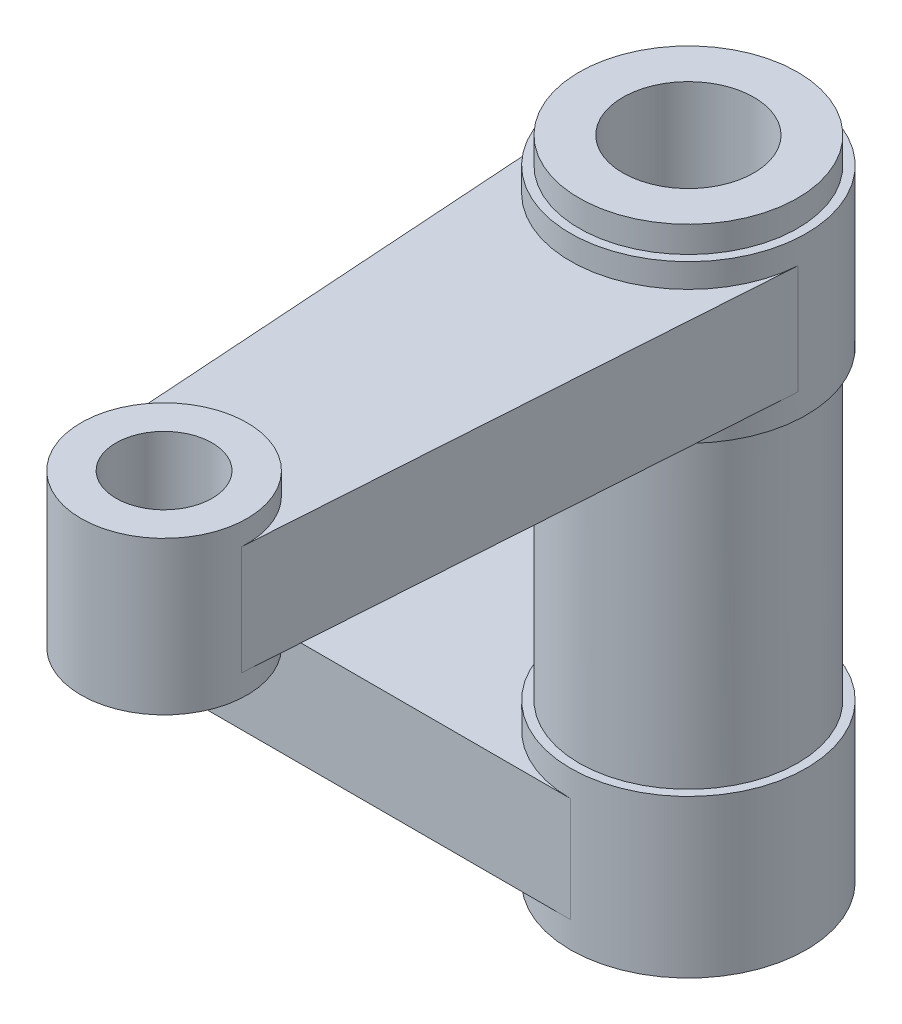
ISO-10303-21;
HEADER;
FILE_DESCRIPTION(('STEP AP214'),'2;1');
FILE_NAME('part.step','',(''),(''),'','','');
FILE_SCHEMA(('AUTOMOTIVE_DESIGN { 1 0 10303 214 1 1 1 1 }'));
ENDSEC;
DATA;
#1=APPLICATION_CONTEXT('core data for automotive mechanical design processes');
#2=APPLICATION_PROTOCOL_DEFINITION('international standard','automotive_design',2000,#1);
#3=PRODUCT_CONTEXT('',#1,'mechanical');
#4=PRODUCT('Part','Part','',(#3));
#5=PRODUCT_RELATED_PRODUCT_CATEGORY('part','',(#4));
#6=PRODUCT_DEFINITION_FORMATION('','',#4);
#7=PRODUCT_DEFINITION_CONTEXT('part definition',#1,'design');
#8=PRODUCT_DEFINITION('design','',#6,#7);
#9=PRODUCT_DEFINITION_SHAPE('','',#8);
#10=(LENGTH_UNIT() NAMED_UNIT(*) SI_UNIT(.MILLI.,.METRE.));
#11=(NAMED_UNIT(*) PLANE_ANGLE_UNIT() SI_UNIT($,.RADIAN.));
#12=(NAMED_UNIT(*) SI_UNIT($,.STERADIAN.) SOLID_ANGLE_UNIT());
#13=UNCERTAINTY_MEASURE_WITH_UNIT(LENGTH_MEASURE(1.E-05),#10,'distance_accuracy_value','');
#14=(GEOMETRIC_REPRESENTATION_CONTEXT(3) GLOBAL_UNCERTAINTY_ASSIGNED_CONTEXT((#13)) GLOBAL_UNIT_ASSIGNED_CONTEXT((#10,
#11,#12)) REPRESENTATION_CONTEXT('',''));
#15=CARTESIAN_POINT('',(0.,0.,0.));
#16=DIRECTION('',(0.,0.,1.));
#17=DIRECTION('',(1.,0.,0.));
#18=AXIS2_PLACEMENT_3D('',#15,#16,#17);
#19=CARTESIAN_POINT('',(-45.,6.,0.));
#20=DIRECTION('',(0.,1.,0.));
#21=DIRECTION('',(0.,0.,1.));
#22=AXIS2_PLACEMENT_3D('',#19,#20,#21);
#23=PLANE('',#22);
#24=CARTESIAN_POINT('',(-45.,6.,0.));
#25=DIRECTION('',(0.,1.,0.));
#26=DIRECTION('',(0.,0.,1.));
#27=AXIS2_PLACEMENT_3D('',#24,#25,#26);
#28=CIRCLE('',#27,7.5);
#29=CARTESIAN_POINT('',(-45.,6.,7.50000000000001));
#30=VERTEX_POINT('',#29);
#31=EDGE_CURVE('E177',#30,#30,#28,.T.);
#32=ORIENTED_EDGE('',*,*,#31,.F.);
#33=EDGE_LOOP('',(#32));
#34=FACE_BOUND('',#33,.T.);
#35=DIRECTION('',(1.,0.,0.));
#36=VECTOR('',#35,1.);
#37=CARTESIAN_POINT('',(-45.,6.,13.5));
#38=LINE('',#37,#36);
#39=CARTESIAN_POINT('',(-45.,6.,13.5));
#40=VERTEX_POINT('',#39);
#41=CARTESIAN_POINT('',(0.,6.,13.5));
#42=VERTEX_POINT('',#41);
#43=EDGE_CURVE('E87',#40,#42,#38,.T.);
#44=ORIENTED_EDGE('',*,*,#43,.T.);
#45=CARTESIAN_POINT('',(0.,6.,0.));
#46=DIRECTION('',(0.,1.,0.));
#47=DIRECTION('',(0.,0.,1.));
#48=AXIS2_PLACEMENT_3D('',#45,#46,#47);
#49=CIRCLE('',#48,13.5);
#50=CARTESIAN_POINT('',(0.,6.,-13.5));
#51=VERTEX_POINT('',#50);
#52=EDGE_CURVE('E180',#42,#51,#49,.F.);
#53=ORIENTED_EDGE('',*,*,#52,.T.);
#54=DIRECTION('',(-1.,0.,0.));
#55=VECTOR('',#54,1.);
#56=CARTESIAN_POINT('',(-45.,6.,-13.5));
#57=LINE('',#56,#55);
#58=CARTESIAN_POINT('',(-45.,6.,-13.5));
#59=VERTEX_POINT('',#58);
#60=EDGE_CURVE('E64',#51,#59,#57,.T.);
#61=ORIENTED_EDGE('',*,*,#60,.T.);
#62=CARTESIAN_POINT('',(-45.,6.,0.));
#63=DIRECTION('',(0.,1.,0.));
#64=DIRECTION('',(0.,0.,1.));
#65=AXIS2_PLACEMENT_3D('',#62,#63,#64);
#66=CIRCLE('',#65,13.5);
#67=EDGE_CURVE('E186',#59,#40,#66,.T.);
#68=ORIENTED_EDGE('',*,*,#67,.T.);
#69=EDGE_LOOP('',(#44,#53,#61,#68));
#70=FACE_BOUND('',#69,.T.);
#71=ADVANCED_FACE('F39',(#34,#70),#23,.T.);
#72=CARTESIAN_POINT('',(-45.,-6.,0.));
#73=DIRECTION('',(0.,1.,0.));
#74=DIRECTION('',(0.,0.,1.));
#75=AXIS2_PLACEMENT_3D('',#72,#73,#74);
#76=PLANE('',#75);
#77=CARTESIAN_POINT('',(-45.,-6.,0.));
#78=DIRECTION('',(0.,1.,0.));
#79=DIRECTION('',(0.,0.,1.));
#80=AXIS2_PLACEMENT_3D('',#77,#78,#79);
#81=CIRCLE('',#80,7.5);
#82=CARTESIAN_POINT('',(-45.,-6.,7.50000000000001));
#83=VERTEX_POINT('',#82);
#84=EDGE_CURVE('E179',#83,#83,#81,.T.);
#85=ORIENTED_EDGE('',*,*,#84,.T.);
#86=EDGE_LOOP('',(#85));
#87=FACE_BOUND('',#86,.T.);
#88=CARTESIAN_POINT('',(0.,-6.,0.));
#89=DIRECTION('',(0.,1.,0.));
#90=DIRECTION('',(0.,0.,1.));
#91=AXIS2_PLACEMENT_3D('',#88,#89,#90);
#92=CIRCLE('',#91,13.5);
#93=CARTESIAN_POINT('',(0.,-6.,13.5));
#94=VERTEX_POINT('',#93);
#95=CARTESIAN_POINT('',(0.,-6.,-13.5));
#96=VERTEX_POINT('',#95);
#97=EDGE_CURVE('E174',#94,#96,#92,.F.);
#98=ORIENTED_EDGE('',*,*,#97,.F.);
#99=DIRECTION('',(1.,0.,0.));
#100=VECTOR('',#99,1.);
#101=CARTESIAN_POINT('',(-45.,-6.,13.5));
#102=LINE('',#101,#100);
#103=CARTESIAN_POINT('',(-45.,-6.,13.5));
#104=VERTEX_POINT('',#103);
#105=EDGE_CURVE('E191',#104,#94,#102,.T.);
#106=ORIENTED_EDGE('',*,*,#105,.F.);
#107=CARTESIAN_POINT('',(-45.,-6.,0.));
#108=DIRECTION('',(0.,1.,0.));
#109=DIRECTION('',(0.,0.,1.));
#110=AXIS2_PLACEMENT_3D('',#107,#108,#109);
#111=CIRCLE('',#110,13.5);
#112=CARTESIAN_POINT('',(-45.,-6.,-13.5));
#113=VERTEX_POINT('',#112);
#114=EDGE_CURVE('E181',#113,#104,#111,.T.);
#115=ORIENTED_EDGE('',*,*,#114,.F.);
#116=DIRECTION('',(-1.,0.,0.));
#117=VECTOR('',#116,1.);
#118=CARTESIAN_POINT('',(-45.,-6.,-13.5));
#119=LINE('',#118,#117);
#120=EDGE_CURVE('E83',#96,#113,#119,.T.);
#121=ORIENTED_EDGE('',*,*,#120,.F.);
#122=EDGE_LOOP('',(#98,#106,#115,#121));
#123=FACE_BOUND('',#122,.T.);
#124=ADVANCED_FACE('F208',(#87,#123),#76,.F.);
#125=CARTESIAN_POINT('',(-45.,6.,0.));
#126=DIRECTION('',(0.,-1.,0.));
#127=DIRECTION('',(0.,0.,-1.));
#128=AXIS2_PLACEMENT_3D('',#125,#126,#127);
#129=CYLINDRICAL_SURFACE('',#128,13.5);
#130=ORIENTED_EDGE('',*,*,#114,.T.);
#131=DIRECTION('',(0.,-1.,0.));
#132=VECTOR('',#131,1.);
#133=CARTESIAN_POINT('',(-45.,6.,13.5));
#134=LINE('',#133,#132);
#135=EDGE_CURVE('E50',#40,#104,#134,.T.);
#136=ORIENTED_EDGE('',*,*,#135,.F.);
#137=ORIENTED_EDGE('',*,*,#67,.F.);
#138=DIRECTION('',(0.,-1.,0.));
#139=VECTOR('',#138,1.);
#140=CARTESIAN_POINT('',(-45.,6.,-13.5));
#141=LINE('',#140,#139);
#142=EDGE_CURVE('E190',#59,#113,#141,.T.);
#143=ORIENTED_EDGE('',*,*,#142,.T.);
#144=EDGE_LOOP('',(#130,#136,#137,#143));
#145=FACE_BOUND('',#144,.T.);
#146=ADVANCED_FACE('F41',(#145),#129,.T.);
#147=CARTESIAN_POINT('',(-45.,6.,13.5));
#148=DIRECTION('',(0.,0.,-1.));
#149=DIRECTION('',(-1.,0.,0.));
#150=AXIS2_PLACEMENT_3D('',#147,#148,#149);
#151=PLANE('',#150);
#152=ORIENTED_EDGE('',*,*,#105,.T.);
#153=DIRECTION('',(0.,-1.,0.));
#154=VECTOR('',#153,1.);
#155=CARTESIAN_POINT('',(0.,6.,13.5));
#156=LINE('',#155,#154);
#157=EDGE_CURVE('E199',#42,#94,#156,.T.);
#158=ORIENTED_EDGE('',*,*,#157,.F.);
#159=ORIENTED_EDGE('',*,*,#43,.F.);
#160=ORIENTED_EDGE('',*,*,#135,.T.);
#161=EDGE_LOOP('',(#152,#158,#159,#160));
#162=FACE_BOUND('',#161,.T.);
#163=ADVANCED_FACE('F201',(#162),#151,.F.);
#164=CARTESIAN_POINT('',(0.,6.,0.));
#165=DIRECTION('',(0.,-1.,0.));
#166=DIRECTION('',(0.,0.,-1.));
#167=AXIS2_PLACEMENT_3D('',#164,#165,#166);
#168=CYLINDRICAL_SURFACE('',#167,13.5);
#169=ORIENTED_EDGE('',*,*,#157,.T.);
#170=ORIENTED_EDGE('',*,*,#97,.T.);
#171=DIRECTION('',(0.,-1.,0.));
#172=VECTOR('',#171,1.);
#173=CARTESIAN_POINT('',(0.,6.,-13.5));
#174=LINE('',#173,#172);
#175=EDGE_CURVE('E196',#51,#96,#174,.T.);
#176=ORIENTED_EDGE('',*,*,#175,.F.);
#177=ORIENTED_EDGE('',*,*,#52,.F.);
#178=EDGE_LOOP('',(#169,#170,#176,#177));
#179=FACE_BOUND('',#178,.T.);
#180=CARTESIAN_POINT('',(0.,-9.,0.));
#181=DIRECTION('',(0.,1.,0.));
#182=DIRECTION('',(0.,0.,1.));
#183=AXIS2_PLACEMENT_3D('',#180,#181,#182);
#184=CIRCLE('',#183,13.5);
#185=CARTESIAN_POINT('',(0.,-9.,13.5));
#186=VERTEX_POINT('',#185);
#187=EDGE_CURVE('E166',#186,#186,#184,.T.);
#188=ORIENTED_EDGE('',*,*,#187,.T.);
#189=EDGE_LOOP('',(#188));
#190=FACE_BOUND('',#189,.T.);
#191=CARTESIAN_POINT('',(0.,9.,0.));
#192=DIRECTION('',(0.,1.,0.));
#193=DIRECTION('',(0.,0.,1.));
#194=AXIS2_PLACEMENT_3D('',#191,#192,#193);
#195=CIRCLE('',#194,13.5);
#196=CARTESIAN_POINT('',(0.,9.,13.5));
#197=VERTEX_POINT('',#196);
#198=EDGE_CURVE('E168',#197,#197,#195,.T.);
#199=ORIENTED_EDGE('',*,*,#198,.F.);
#200=EDGE_LOOP('',(#199));
#201=FACE_BOUND('',#200,.T.);
#202=ADVANCED_FACE('F211',(#179,#190,#201),#168,.T.);
#203=CARTESIAN_POINT('',(-45.,6.,-13.5));
#204=DIRECTION('',(0.,0.,1.));
#205=DIRECTION('',(1.,0.,0.));
#206=AXIS2_PLACEMENT_3D('',#203,#204,#205);
#207=PLANE('',#206);
#208=ORIENTED_EDGE('',*,*,#120,.T.);
#209=ORIENTED_EDGE('',*,*,#142,.F.);
#210=ORIENTED_EDGE('',*,*,#60,.F.);
#211=ORIENTED_EDGE('',*,*,#175,.T.);
#212=EDGE_LOOP('',(#208,#209,#210,#211));
#213=FACE_BOUND('',#212,.T.);
#214=ADVANCED_FACE('F212',(#213),#207,.F.);
#215=CARTESIAN_POINT('',(-45.,6.,0.));
#216=DIRECTION('',(0.,-1.,0.));
#217=DIRECTION('',(0.,0.,-1.));
#218=AXIS2_PLACEMENT_3D('',#215,#216,#217);
#219=CYLINDRICAL_SURFACE('',#218,7.5);
#220=ORIENTED_EDGE('',*,*,#31,.T.);
#221=EDGE_LOOP('',(#220));
#222=FACE_BOUND('',#221,.T.);
#223=ORIENTED_EDGE('',*,*,#84,.F.);
#224=EDGE_LOOP('',(#223));
#225=FACE_BOUND('',#224,.T.);
#226=ADVANCED_FACE('F226',(#222,#225),#219,.F.);
#227=CARTESIAN_POINT('',(0.,-9.,0.));
#228=DIRECTION('',(0.,1.,0.));
#229=DIRECTION('',(0.,0.,1.));
#230=AXIS2_PLACEMENT_3D('',#227,#228,#229);
#231=PLANE('',#230);
#232=CARTESIAN_POINT('',(0.,-8.99999999999999,0.));
#233=DIRECTION('',(0.,1.,0.));
#234=DIRECTION('',(0.,0.,1.));
#235=AXIS2_PLACEMENT_3D('',#232,#233,#234);
#236=CIRCLE('',#235,7.5);
#237=CARTESIAN_POINT('',(0.,-8.99999999999999,7.5));
#238=VERTEX_POINT('',#237);
#239=EDGE_CURVE('E149',#238,#238,#236,.T.);
#240=ORIENTED_EDGE('',*,*,#239,.T.);
#241=EDGE_LOOP('',(#240));
#242=FACE_BOUND('',#241,.T.);
#243=ORIENTED_EDGE('',*,*,#187,.F.);
#244=EDGE_LOOP('',(#243));
#245=FACE_BOUND('',#244,.T.);
#246=ADVANCED_FACE('F244',(#242,#245),#231,.F.);
#247=CARTESIAN_POINT('',(0.,9.,0.));
#248=DIRECTION('',(0.,1.,0.));
#249=DIRECTION('',(0.,0.,1.));
#250=AXIS2_PLACEMENT_3D('',#247,#248,#249);
#251=PLANE('',#250);
#252=CARTESIAN_POINT('',(0.,9.,0.));
#253=DIRECTION('',(0.,1.,0.));
#254=DIRECTION('',(0.,0.,1.));
#255=AXIS2_PLACEMENT_3D('',#252,#253,#254);
#256=CIRCLE('',#255,12.5);
#257=CARTESIAN_POINT('',(0.,9.,12.5));
#258=VERTEX_POINT('',#257);
#259=EDGE_CURVE('E11',#258,#258,#256,.T.);
#260=ORIENTED_EDGE('',*,*,#259,.F.);
#261=EDGE_LOOP('',(#260));
#262=FACE_BOUND('',#261,.T.);
#263=ORIENTED_EDGE('',*,*,#198,.T.);
#264=EDGE_LOOP('',(#263));
#265=FACE_BOUND('',#264,.T.);
#266=ADVANCED_FACE('F277',(#262,#265),#251,.T.);
#267=CARTESIAN_POINT('',(0.,65.,0.));
#268=DIRECTION('',(0.,1.,0.));
#269=DIRECTION('',(0.,0.,1.));
#270=AXIS2_PLACEMENT_3D('',#267,#268,#269);
#271=PLANE('',#270);
#272=CARTESIAN_POINT('',(0.,65.,0.));
#273=DIRECTION('',(0.,1.,0.));
#274=DIRECTION('',(0.,0.,1.));
#275=AXIS2_PLACEMENT_3D('',#272,#273,#274);
#276=CIRCLE('',#275,7.5);
#277=CARTESIAN_POINT('',(0.,65.,7.5));
#278=VERTEX_POINT('',#277);
#279=EDGE_CURVE('E146',#278,#278,#276,.T.);
#280=ORIENTED_EDGE('',*,*,#279,.F.);
#281=EDGE_LOOP('',(#280));
#282=FACE_BOUND('',#281,.T.);
#283=CARTESIAN_POINT('',(0.,65.,0.));
#284=DIRECTION('',(0.,-1.,0.));
#285=DIRECTION('',(0.,0.,-1.));
#286=AXIS2_PLACEMENT_3D('',#283,#284,#285);
#287=CIRCLE('',#286,12.5);
#288=CARTESIAN_POINT('',(0.,65.,-12.5));
#289=VERTEX_POINT('',#288);
#290=EDGE_CURVE('E167',#289,#289,#287,.T.);
#291=ORIENTED_EDGE('',*,*,#290,.F.);
#292=EDGE_LOOP('',(#291));
#293=FACE_BOUND('',#292,.T.);
#294=ADVANCED_FACE('F290',(#282,#293),#271,.T.);
#295=CARTESIAN_POINT('',(0.,0.,0.));
#296=DIRECTION('',(0.,-1.,0.));
#297=DIRECTION('',(0.,0.,-1.));
#298=AXIS2_PLACEMENT_3D('',#295,#296,#297);
#299=CYLINDRICAL_SURFACE('',#298,12.5);
#300=ORIENTED_EDGE('',*,*,#290,.T.);
#301=EDGE_LOOP('',(#300));
#302=FACE_BOUND('',#301,.T.);
#303=CARTESIAN_POINT('',(0.,62.,0.));
#304=DIRECTION('',(0.,-1.,0.));
#305=DIRECTION('',(0.,0.,-1.));
#306=AXIS2_PLACEMENT_3D('',#303,#304,#305);
#307=CIRCLE('',#306,12.5);
#308=CARTESIAN_POINT('',(0.,62.,-12.5));
#309=VERTEX_POINT('',#308);
#310=EDGE_CURVE('E162',#309,#309,#307,.T.);
#311=ORIENTED_EDGE('',*,*,#310,.F.);
#312=EDGE_LOOP('',(#311));
#313=FACE_BOUND('',#312,.T.);
#314=ADVANCED_FACE('F297',(#302,#313),#299,.T.);
#315=CARTESIAN_POINT('',(12.5,62.,0.));
#316=DIRECTION('',(0.,1.,0.));
#317=DIRECTION('',(0.,0.,1.));
#318=AXIS2_PLACEMENT_3D('',#315,#316,#317);
#319=PLANE('',#318);
#320=ORIENTED_EDGE('',*,*,#310,.T.);
#321=EDGE_LOOP('',(#320));
#322=FACE_BOUND('',#321,.T.);
#323=CARTESIAN_POINT('',(0.,62.,0.));
#324=DIRECTION('',(0.,-1.,0.));
#325=DIRECTION('',(0.,0.,-1.));
#326=AXIS2_PLACEMENT_3D('',#323,#324,#325);
#327=CIRCLE('',#326,13.5);
#328=CARTESIAN_POINT('',(0.,62.,-13.5));
#329=VERTEX_POINT('',#328);
#330=EDGE_CURVE('E159',#329,#329,#327,.T.);
#331=ORIENTED_EDGE('',*,*,#330,.F.);
#332=EDGE_LOOP('',(#331));
#333=FACE_BOUND('',#332,.T.);
#334=ADVANCED_FACE('F307',(#322,#333),#319,.T.);
#335=CARTESIAN_POINT('',(0.,0.,0.));
#336=DIRECTION('',(0.,-1.,0.));
#337=DIRECTION('',(0.,0.,-1.));
#338=AXIS2_PLACEMENT_3D('',#335,#336,#337);
#339=CYLINDRICAL_SURFACE('',#338,13.5);
#340=CARTESIAN_POINT('',(0.,59.25,0.));
#341=DIRECTION('',(0.,-1.,0.));
#342=DIRECTION('',(0.,0.,1.));
#343=AXIS2_PLACEMENT_3D('',#340,#341,#342);
#344=CIRCLE('',#343,13.5);
#345=CARTESIAN_POINT('',(13.4699665923862,59.25,0.899999999999999));
#346=VERTEX_POINT('',#345);
#347=CARTESIAN_POINT('',(-13.4699665923862,59.25,0.900000000000002));
#348=VERTEX_POINT('',#347);
#349=EDGE_CURVE('E122',#346,#348,#344,.T.);
#350=ORIENTED_EDGE('',*,*,#349,.F.);
#351=DIRECTION('',(0.,-1.,0.));
#352=VECTOR('',#351,1.);
#353=CARTESIAN_POINT('',(13.4699665923862,59.25,0.899999999999999));
#354=LINE('',#353,#352);
#355=CARTESIAN_POINT('',(13.4699665923862,46.75,0.899999999999999));
#356=VERTEX_POINT('',#355);
#357=EDGE_CURVE('E135',#346,#356,#354,.T.);
#358=ORIENTED_EDGE('',*,*,#357,.T.);
#359=CARTESIAN_POINT('',(0.,46.75,0.));
#360=DIRECTION('',(0.,-1.,0.));
#361=DIRECTION('',(0.,0.,1.));
#362=AXIS2_PLACEMENT_3D('',#359,#360,#361);
#363=CIRCLE('',#362,13.5);
#364=CARTESIAN_POINT('',(-13.4699665923862,46.75,0.900000000000002));
#365=VERTEX_POINT('',#364);
#366=EDGE_CURVE('E123',#356,#365,#363,.T.);
#367=ORIENTED_EDGE('',*,*,#366,.T.);
#368=DIRECTION('',(0.,-1.,0.));
#369=VECTOR('',#368,1.);
#370=CARTESIAN_POINT('',(-13.4699665923862,59.25,0.900000000000002));
#371=LINE('',#370,#369);
#372=EDGE_CURVE('E53',#348,#365,#371,.T.);
#373=ORIENTED_EDGE('',*,*,#372,.F.);
#374=EDGE_LOOP('',(#350,#358,#367,#373));
#375=FACE_BOUND('',#374,.T.);
#376=ORIENTED_EDGE('',*,*,#330,.T.);
#377=EDGE_LOOP('',(#376));
#378=FACE_BOUND('',#377,.T.);
#379=CARTESIAN_POINT('',(0.,44.,0.));
#380=DIRECTION('',(0.,-1.,0.));
#381=DIRECTION('',(0.,0.,-1.));
#382=AXIS2_PLACEMENT_3D('',#379,#380,#381);
#383=CIRCLE('',#382,13.5);
#384=CARTESIAN_POINT('',(0.,44.,-13.5));
#385=VERTEX_POINT('',#384);
#386=EDGE_CURVE('E160',#385,#385,#383,.T.);
#387=ORIENTED_EDGE('',*,*,#386,.F.);
#388=EDGE_LOOP('',(#387));
#389=FACE_BOUND('',#388,.T.);
#390=ADVANCED_FACE('F320',(#375,#378,#389),#339,.T.);
#391=CARTESIAN_POINT('',(13.5,44.,0.));
#392=DIRECTION('',(0.,-1.,0.));
#393=DIRECTION('',(0.,0.,-1.));
#394=AXIS2_PLACEMENT_3D('',#391,#392,#393);
#395=PLANE('',#394);
#396=ORIENTED_EDGE('',*,*,#386,.T.);
#397=EDGE_LOOP('',(#396));
#398=FACE_BOUND('',#397,.T.);
#399=CARTESIAN_POINT('',(0.,44.,0.));
#400=DIRECTION('',(0.,-1.,0.));
#401=DIRECTION('',(0.,0.,-1.));
#402=AXIS2_PLACEMENT_3D('',#399,#400,#401);
#403=CIRCLE('',#402,12.5);
#404=CARTESIAN_POINT('',(0.,44.,-12.5));
#405=VERTEX_POINT('',#404);
#406=EDGE_CURVE('E155',#405,#405,#403,.T.);
#407=ORIENTED_EDGE('',*,*,#406,.F.);
#408=EDGE_LOOP('',(#407));
#409=FACE_BOUND('',#408,.T.);
#410=ADVANCED_FACE('F327',(#398,#409),#395,.T.);
#411=CARTESIAN_POINT('',(0.,0.,0.));
#412=DIRECTION('',(0.,-1.,0.));
#413=DIRECTION('',(0.,0.,-1.));
#414=AXIS2_PLACEMENT_3D('',#411,#412,#413);
#415=CYLINDRICAL_SURFACE('',#414,12.5);
#416=ORIENTED_EDGE('',*,*,#259,.T.);
#417=EDGE_LOOP('',(#416));
#418=FACE_BOUND('',#417,.T.);
#419=ORIENTED_EDGE('',*,*,#406,.T.);
#420=EDGE_LOOP('',(#419));
#421=FACE_BOUND('',#420,.T.);
#422=ADVANCED_FACE('F339',(#418,#421),#415,.T.);
#423=CARTESIAN_POINT('',(0.,-8.99999999999999,0.));
#424=DIRECTION('',(0.,1.,0.));
#425=DIRECTION('',(0.,0.,1.));
#426=AXIS2_PLACEMENT_3D('',#423,#424,#425);
#427=CYLINDRICAL_SURFACE('',#426,7.5);
#428=ORIENTED_EDGE('',*,*,#239,.F.);
#429=EDGE_LOOP('',(#428));
#430=FACE_BOUND('',#429,.T.);
#431=ORIENTED_EDGE('',*,*,#279,.T.);
#432=EDGE_LOOP('',(#431));
#433=FACE_BOUND('',#432,.T.);
#434=ADVANCED_FACE('F350',(#430,#433),#427,.F.);
#435=CARTESIAN_POINT('',(-13.4699665923862,59.25,0.900000000000002));
#436=DIRECTION('',(0.997775303139718,0.,-0.0666666666666668));
#437=DIRECTION('',(-0.0666666666666668,0.,-0.997775303139718));
#438=AXIS2_PLACEMENT_3D('',#435,#436,#437);
#439=PLANE('',#438);
#440=DIRECTION('',(0.0666666666666668,0.,0.997775303139718));
#441=VECTOR('',#440,1.);
#442=CARTESIAN_POINT('',(-13.4699665923862,46.75,0.900000000000002));
#443=LINE('',#442,#441);
#444=CARTESIAN_POINT('',(-9.47886537982732,46.75,60.6333333333333));
#445=VERTEX_POINT('',#444);
#446=EDGE_CURVE('E137',#365,#445,#443,.T.);
#447=ORIENTED_EDGE('',*,*,#446,.T.);
#448=DIRECTION('',(0.,-1.,0.));
#449=VECTOR('',#448,1.);
#450=CARTESIAN_POINT('',(-9.47886537982732,59.25,60.6333333333333));
#451=LINE('',#450,#449);
#452=CARTESIAN_POINT('',(-9.47886537982732,59.25,60.6333333333333));
#453=VERTEX_POINT('',#452);
#454=EDGE_CURVE('E133',#453,#445,#451,.T.);
#455=ORIENTED_EDGE('',*,*,#454,.F.);
#456=DIRECTION('',(0.0666666666666668,0.,0.997775303139718));
#457=VECTOR('',#456,1.);
#458=CARTESIAN_POINT('',(-13.4699665923862,59.25,0.900000000000002));
#459=LINE('',#458,#457);
#460=EDGE_CURVE('E433',#348,#453,#459,.T.);
#461=ORIENTED_EDGE('',*,*,#460,.F.);
#462=ORIENTED_EDGE('',*,*,#372,.T.);
#463=EDGE_LOOP('',(#447,#455,#461,#462));
#464=FACE_BOUND('',#463,.T.);
#465=ADVANCED_FACE('F358',(#464),#439,.F.);
#466=CARTESIAN_POINT('',(13.4699665923862,59.25,0.899999999999999));
#467=DIRECTION('',(-0.997775303139718,0.,-0.0666666666666666));
#468=DIRECTION('',(-0.0666666666666666,0.,0.997775303139718));
#469=AXIS2_PLACEMENT_3D('',#466,#467,#468);
#470=PLANE('',#469);
#471=DIRECTION('',(0.0666666666666666,0.,-0.997775303139718));
#472=VECTOR('',#471,1.);
#473=CARTESIAN_POINT('',(13.4699665923862,46.75,0.899999999999999));
#474=LINE('',#473,#472);
#475=CARTESIAN_POINT('',(9.47886537982733,46.75,60.6333333333333));
#476=VERTEX_POINT('',#475);
#477=EDGE_CURVE('E111',#476,#356,#474,.T.);
#478=ORIENTED_EDGE('',*,*,#477,.T.);
#479=ORIENTED_EDGE('',*,*,#357,.F.);
#480=DIRECTION('',(0.0666666666666666,0.,-0.997775303139718));
#481=VECTOR('',#480,1.);
#482=CARTESIAN_POINT('',(13.4699665923862,59.25,0.899999999999999));
#483=LINE('',#482,#481);
#484=CARTESIAN_POINT('',(9.47886537982733,59.25,60.6333333333333));
#485=VERTEX_POINT('',#484);
#486=EDGE_CURVE('E131',#485,#346,#483,.T.);
#487=ORIENTED_EDGE('',*,*,#486,.F.);
#488=DIRECTION('',(0.,-1.,0.));
#489=VECTOR('',#488,1.);
#490=CARTESIAN_POINT('',(9.47886537982733,59.25,60.6333333333333));
#491=LINE('',#490,#489);
#492=EDGE_CURVE('E129',#485,#476,#491,.T.);
#493=ORIENTED_EDGE('',*,*,#492,.T.);
#494=EDGE_LOOP('',(#478,#479,#487,#493));
#495=FACE_BOUND('',#494,.T.);
#496=ADVANCED_FACE('F128',(#495),#470,.F.);
#497=CARTESIAN_POINT('',(0.,59.25,0.));
#498=DIRECTION('',(0.,1.,0.));
#499=DIRECTION('',(0.,0.,1.));
#500=AXIS2_PLACEMENT_3D('',#497,#498,#499);
#501=PLANE('',#500);
#502=ORIENTED_EDGE('',*,*,#349,.T.);
#503=ORIENTED_EDGE('',*,*,#460,.T.);
#504=CARTESIAN_POINT('',(0.,59.25,60.));
#505=DIRECTION('',(0.,-1.,0.));
#506=DIRECTION('',(0.,0.,1.));
#507=AXIS2_PLACEMENT_3D('',#504,#505,#506);
#508=CIRCLE('',#507,9.5);
#509=EDGE_CURVE('E445',#453,#485,#508,.T.);
#510=ORIENTED_EDGE('',*,*,#509,.T.);
#511=ORIENTED_EDGE('',*,*,#486,.T.);
#512=EDGE_LOOP('',(#502,#503,#510,#511));
#513=FACE_BOUND('',#512,.T.);
#514=ADVANCED_FACE('F407',(#513),#501,.T.);
#515=CARTESIAN_POINT('',(0.,46.75,0.));
#516=DIRECTION('',(0.,1.,0.));
#517=DIRECTION('',(0.,0.,1.));
#518=AXIS2_PLACEMENT_3D('',#515,#516,#517);
#519=PLANE('',#518);
#520=ORIENTED_EDGE('',*,*,#366,.F.);
#521=ORIENTED_EDGE('',*,*,#477,.F.);
#522=CARTESIAN_POINT('',(0.,46.75,60.));
#523=DIRECTION('',(0.,-1.,0.));
#524=DIRECTION('',(0.,0.,1.));
#525=AXIS2_PLACEMENT_3D('',#522,#523,#524);
#526=CIRCLE('',#525,9.5);
#527=EDGE_CURVE('E119',#445,#476,#526,.T.);
#528=ORIENTED_EDGE('',*,*,#527,.F.);
#529=ORIENTED_EDGE('',*,*,#446,.F.);
#530=EDGE_LOOP('',(#520,#521,#528,#529));
#531=FACE_BOUND('',#530,.T.);
#532=ADVANCED_FACE('F116',(#531),#519,.F.);
#533=CARTESIAN_POINT('',(0.,61.75,60.));
#534=DIRECTION('',(0.,1.,0.));
#535=DIRECTION('',(0.,0.,1.));
#536=AXIS2_PLACEMENT_3D('',#533,#534,#535);
#537=PLANE('',#536);
#538=CARTESIAN_POINT('',(0.,61.75,60.));
#539=DIRECTION('',(0.,1.,0.));
#540=DIRECTION('',(0.,0.,1.));
#541=AXIS2_PLACEMENT_3D('',#538,#539,#540);
#542=CIRCLE('',#541,9.5);
#543=CARTESIAN_POINT('',(0.,61.75,69.5));
#544=VERTEX_POINT('',#543);
#545=EDGE_CURVE('E436',#544,#544,#542,.T.);
#546=ORIENTED_EDGE('',*,*,#545,.T.);
#547=EDGE_LOOP('',(#546));
#548=FACE_BOUND('',#547,.T.);
#549=CARTESIAN_POINT('',(0.,61.75,60.));
#550=DIRECTION('',(0.,1.,0.));
#551=DIRECTION('',(0.,0.,1.));
#552=AXIS2_PLACEMENT_3D('',#549,#550,#551);
#553=CIRCLE('',#552,5.5);
#554=CARTESIAN_POINT('',(0.,61.75,65.5));
#555=VERTEX_POINT('',#554);
#556=EDGE_CURVE('E446',#555,#555,#553,.T.);
#557=ORIENTED_EDGE('',*,*,#556,.F.);
#558=EDGE_LOOP('',(#557));
#559=FACE_BOUND('',#558,.T.);
#560=ADVANCED_FACE('F362',(#548,#559),#537,.T.);
#561=CARTESIAN_POINT('',(0.,44.25,60.));
#562=DIRECTION('',(0.,1.,0.));
#563=DIRECTION('',(0.,0.,1.));
#564=AXIS2_PLACEMENT_3D('',#561,#562,#563);
#565=PLANE('',#564);
#566=CARTESIAN_POINT('',(0.,44.25,60.));
#567=DIRECTION('',(0.,1.,0.));
#568=DIRECTION('',(0.,0.,1.));
#569=AXIS2_PLACEMENT_3D('',#566,#567,#568);
#570=CIRCLE('',#569,9.5);
#571=CARTESIAN_POINT('',(0.,44.25,69.5));
#572=VERTEX_POINT('',#571);
#573=EDGE_CURVE('E437',#572,#572,#570,.T.);
#574=ORIENTED_EDGE('',*,*,#573,.F.);
#575=EDGE_LOOP('',(#574));
#576=FACE_BOUND('',#575,.T.);
#577=CARTESIAN_POINT('',(0.,44.25,60.));
#578=DIRECTION('',(0.,1.,0.));
#579=DIRECTION('',(0.,0.,1.));
#580=AXIS2_PLACEMENT_3D('',#577,#578,#579);
#581=CIRCLE('',#580,5.5);
#582=CARTESIAN_POINT('',(0.,44.25,65.5));
#583=VERTEX_POINT('',#582);
#584=EDGE_CURVE('E449',#583,#583,#581,.T.);
#585=ORIENTED_EDGE('',*,*,#584,.T.);
#586=EDGE_LOOP('',(#585));
#587=FACE_BOUND('',#586,.T.);
#588=ADVANCED_FACE('F370',(#576,#587),#565,.F.);
#589=CARTESIAN_POINT('',(0.,61.75,60.));
#590=DIRECTION('',(0.,-1.,0.));
#591=DIRECTION('',(0.,0.,-1.));
#592=AXIS2_PLACEMENT_3D('',#589,#590,#591);
#593=CYLINDRICAL_SURFACE('',#592,9.5);
#594=ORIENTED_EDGE('',*,*,#509,.F.);
#595=ORIENTED_EDGE('',*,*,#454,.T.);
#596=ORIENTED_EDGE('',*,*,#527,.T.);
#597=ORIENTED_EDGE('',*,*,#492,.F.);
#598=EDGE_LOOP('',(#594,#595,#596,#597));
#599=FACE_BOUND('',#598,.T.);
#600=ORIENTED_EDGE('',*,*,#545,.F.);
#601=EDGE_LOOP('',(#600));
#602=FACE_BOUND('',#601,.T.);
#603=ORIENTED_EDGE('',*,*,#573,.T.);
#604=EDGE_LOOP('',(#603));
#605=FACE_BOUND('',#604,.T.);
#606=ADVANCED_FACE('F140',(#599,#602,#605),#593,.T.);
#607=CARTESIAN_POINT('',(0.,61.75,60.));
#608=DIRECTION('',(0.,-1.,0.));
#609=DIRECTION('',(0.,0.,-1.));
#610=AXIS2_PLACEMENT_3D('',#607,#608,#609);
#611=CYLINDRICAL_SURFACE('',#610,5.5);
#612=ORIENTED_EDGE('',*,*,#556,.T.);
#613=EDGE_LOOP('',(#612));
#614=FACE_BOUND('',#613,.T.);
#615=ORIENTED_EDGE('',*,*,#584,.F.);
#616=EDGE_LOOP('',(#615));
#617=FACE_BOUND('',#616,.T.);
#618=ADVANCED_FACE('F383',(#614,#617),#611,.F.);
#619=CLOSED_SHELL('',(#71,#124,#146,#163,#202,#214,#226,#246,#266,#294,#314,#334,#390,#410,#422,
#434,#465,#496,#514,#532,#560,#588,#606,#618));
#620=MANIFOLD_SOLID_BREP('B2',#619);
#621=ADVANCED_BREP_SHAPE_REPRESENTATION('',(#18,#620),#14);
#622=SHAPE_DEFINITION_REPRESENTATION(#9,#621);
ENDSEC;
END-ISO-10303-21;
